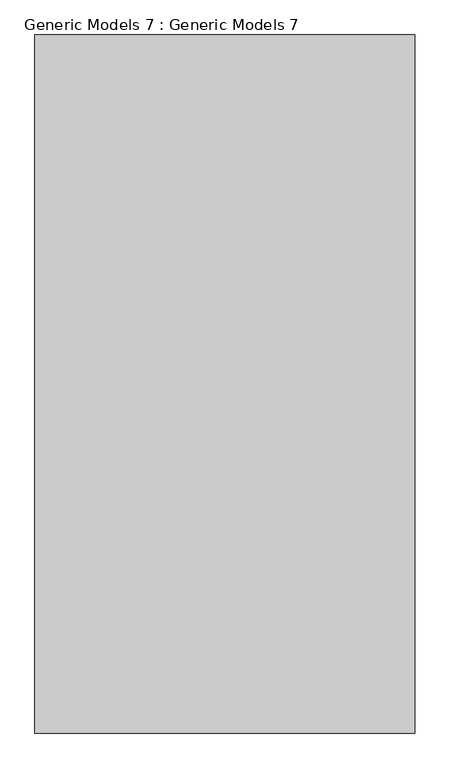
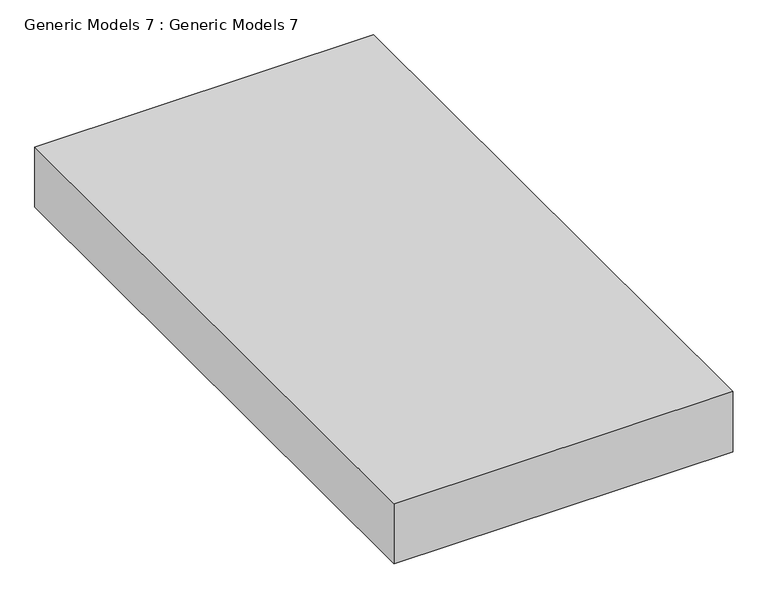
"""IFC4 building model written with IfcOpenShell, lengths in millimetres: proxy geometry, Generic Models 7 : Generic Models 7."""

from ifc_helpers import new_model, si_unit, frame, origin, place, context, project, spatial, polyline, outline, extrude, source, transform, mapped, element, save


def generic_models_7_generic_models_7_82613ab6(model_context):
    return source(origin(), model_context, "Body", "SweptSolid", [
        extrude(outline(polyline([(-21035.2120831, -9098.7538033), (-19816.0120831, -9098.7538033), (-19816.0120831, -11338.5945627), (-21035.2120831, -11338.5945627), (-21035.2120831, -9098.7538033)])), frame((0.0, 0.0, 2481.0176056), z_axis=(0.0, 0.0, 1.0), x_axis=(1.0, 0.0, 0.0)), (0.0, 0.0, 1.0), 228.6),
    ])


if __name__ == "__main__":
    model = new_model("IFC4")
    model_context = context("Model", 3, world=origin())
    ifc_project = project(units=[si_unit("LENGTHUNIT", "METRE", prefix="MILLI")], contexts=[model_context])
    site = spatial("IfcSite", under=ifc_project)
    building = spatial("IfcBuilding", under=site)
    placement = place(None, origin())
    generic_models_7_generic_models_7_shape = generic_models_7_generic_models_7_82613ab6(model_context)
    element("IfcBuildingElementProxy", 1, Name="Generic Models 7 : Generic Models 7", ObjectType="Generic Models 7 : Generic Models 7", at=placement, inside=building, context=model_context, shape_type="MappedRepresentation", body=[
        mapped(generic_models_7_generic_models_7_shape, transform((0.0, 0.0, 0.0), x_axis=(1.0, 0.0, 0.0), y_axis=(0.0, 1.0, 0.0), z_axis=(0.0, 0.0, 1.0))),
    ])
    save(model, "model.ifc")
